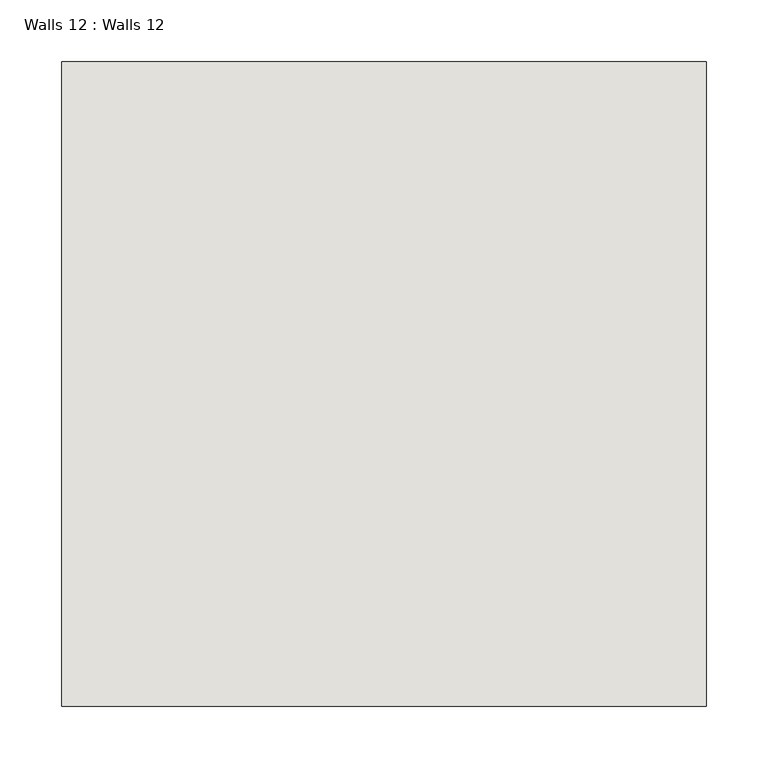
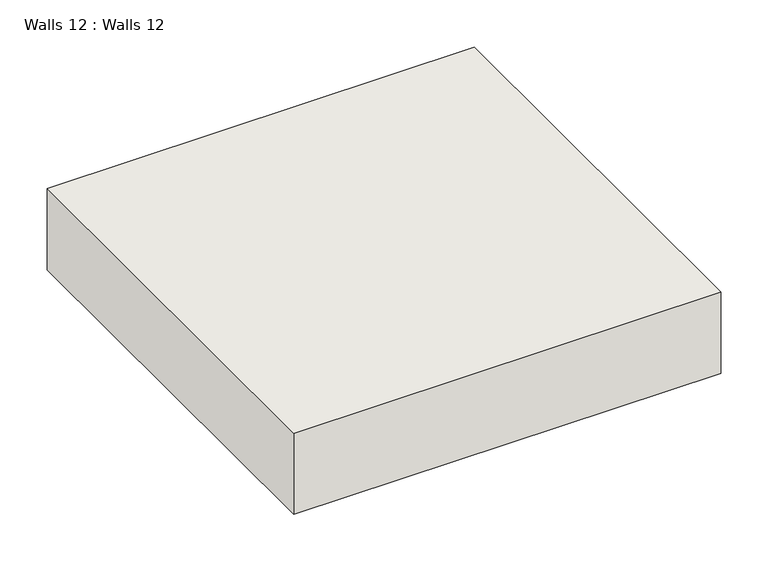
"""IFC4 building model written with IfcOpenShell, lengths in millimetres: wall geometry, Walls 12 : Walls 12."""

from ifc_helpers import new_model, si_unit, frame, origin, place, context, project, spatial, polyline, outline, extrude, source, transform, mapped, element, save


def walls_12_walls_12_bacc6a5f(model_context):
    return source(origin(), model_context, "Body", "SweptSolid", [
        extrude(outline(polyline([(-7406.1805193, -4647.6713241), (-7926.8805193, -4647.6713241), (-7926.8805193, -4126.9713241), (-7406.1805193, -4126.9713241), (-7406.1805193, -4647.6713241)])), frame((0.0, 0.0, 2133.6), z_axis=(0.0, 0.0, 1.0), x_axis=(1.0, 0.0, 0.0)), (0.0, 0.0, 1.0), 104.8762222),
    ])


if __name__ == "__main__":
    model = new_model("IFC4")
    model_context = context("Model", 3, world=origin())
    ifc_project = project(units=[si_unit("LENGTHUNIT", "METRE", prefix="MILLI")], contexts=[model_context])
    site = spatial("IfcSite", under=ifc_project)
    building = spatial("IfcBuilding", under=site)
    placement = place(None, origin())
    walls_12_walls_12_shape = walls_12_walls_12_bacc6a5f(model_context)
    element("IfcWall", 1, ObjectType="Walls 12 : Walls 12", at=placement, inside=building, context=model_context, shape_type="MappedRepresentation", body=[
        mapped(walls_12_walls_12_shape, transform((0.0, 0.0, 0.0), x_axis=(1.0, 0.0, 0.0), y_axis=(0.0, 1.0, 0.0), z_axis=(0.0, 0.0, 1.0))),
    ])
    save(model, "model.ifc")

# Revit data of these elements
# Element 1 (IfcWall, "Walls 12 : Walls 12")
#   Materials on its faces: "Default Wall"
# Materials
#   "Default Wall": colour RGB 128 128 128, transparency 0
